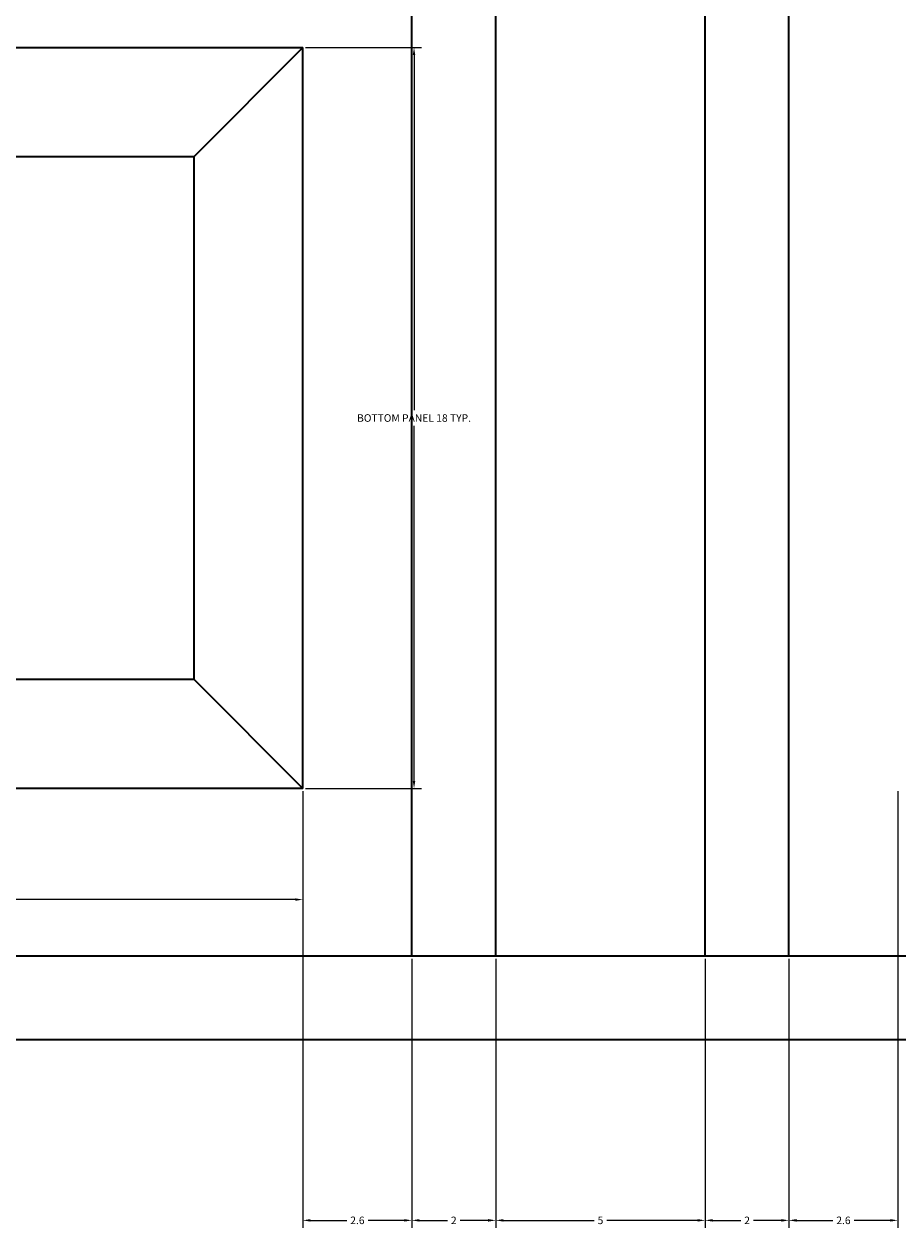
# Model space of a CAD drawing. Units: inches. Extents: x 3137 to 3299, y 1994 to 2089.
# Tile 9 of 14: x 3251 to 3272, y 1996 to 2024. Entities that reach past the tile are written whole.
import ezdxf

# ---------------------------------------------------------------- set-up
doc = ezdxf.new("R2010")
doc.units = ezdxf.units.IN
doc.header["$MEASUREMENT"] = 0
doc.layers.add('A-ANNO-DIMS', color=2, linetype='Continuous', lineweight=18)
doc.layers.add('A-DOOR', color=4, linetype='Continuous', lineweight=35)
doc.styles.get("Standard").update_dxf_attribs({"font": 'arial.ttf'})
doc.dimstyles.get("Standard").update_dxf_attribs({"dimtxt": 0.18, "dimasz": 0.18, "dimexe": 0.18, "dimexo": 0.0625, "dimgap": 0.09, "dimtad": 0, "dimtih": 1, "dimtoh": 1, "dimdec": 4, "dimzin": 0, "dimdsep": 46, "dimtxsty": 'Standard', "dimcen": 0.09, "dimadec": 0, "dimazin": 0, "dimtfac": 1, "dimtdec": 4, "dimtofl": 0, "dimtmove": 0, "dimatfit": 3, "dimfxl": 1, "dimtolj": 1, "dimtzin": 0, "dimarcsym": 0})

# ---------------------------------------------------------------- blocks, each defined once
blk = doc.blocks.new('DOOR-PANEL-RAISED-BOT')
for p, q in [((0, 17.675), (16.9, 17.675)), ((2.6, 15.075), (0, 17.675)), ((14.3, 15.075), (16.9, 17.675)), ((16.9, 0), (16.9, 17.675)), ((2.6, 15.075), (14.3, 15.075)), ((14.3, 2.6), (14.3, 15.075)), ((2.6, 2.6), (0, 0)), ((14.3, 2.6), (16.9, 0))]:
    blk.add_line(p, q)
for points in [[(16.9, 0), (0, 0), (0, 17.675)], [(14.3, 2.6), (2.6, 2.6), (2.6, 15.075)]]:
    blk.add_lwpolyline(points)
blk = doc.blocks.new('*D9')
at = {"layer": 'A-ANNO-DIMS', "color": 0, "lineweight": -2, "transparency": 16777216}
for p, q in [((3257.466, 2023.851), (3260.235, 2023.851)), ((3260.055, 2023.671), (3260.055, 2015.197)), ((3260.055, 2006.356), (3260.055, 2014.83)), ((3257.466, 2006.176), (3260.235, 2006.176))]:
    blk.add_line(p, q, dxfattribs=at)
at = {"layer": 'A-ANNO-DIMS', "color": 0, "transparency": 16777216}
for points in [[(3260.025, 2023.671), (3260.085, 2023.671), (3260.055, 2023.851)], [(3260.025, 2006.356), (3260.085, 2006.356), (3260.055, 2006.176)]]:
    blk.add_solid(points, dxfattribs=at)
at = {"layer": 'Defpoints', "color": 0, "transparency": 16777216}
for p in [(3257.404, 2023.851), (3260.055, 2023.851), (3257.404, 2006.176)]:
    blk.add_point(p, dxfattribs=at)
at = {"layer": 'A-ANNO-DIMS', "color": 0, "transparency": 16777216, "insert": (3260.055, 2015.013), "char_height": 0.18, "attachment_point": 5}
blk.add_mtext('\\A1;BOTTOM PANEL 18 TYP.', dxfattribs=at)
blk = doc.blocks.new('*D10')
at = {"layer": 'A-ANNO-DIMS', "color": 0, "lineweight": -2, "transparency": 16777216}
for p, q in [((3240.504, 2006.113), (3240.504, 2003.344)), ((3257.404, 2006.113), (3257.404, 2003.344)), ((3240.684, 2003.524), (3248.434, 2003.524)), ((3257.224, 2003.524), (3249.474, 2003.524))]:
    blk.add_line(p, q, dxfattribs=at)
at = {"layer": 'A-ANNO-DIMS', "color": 0, "transparency": 16777216}
for points in [[(3240.684, 2003.554), (3240.684, 2003.494), (3240.504, 2003.524)], [(3257.224, 2003.554), (3257.224, 2003.494), (3257.404, 2003.524)]]:
    blk.add_solid(points, dxfattribs=at)
at = {"layer": 'Defpoints', "color": 0, "transparency": 16777216}
for p in [(3240.504, 2006.176), (3257.404, 2006.176), (3257.404, 2003.524)]:
    blk.add_point(p, dxfattribs=at)
at = {"layer": 'A-ANNO-DIMS', "color": 0, "transparency": 16777216, "insert": (3248.954, 2003.524), "char_height": 0.18, "attachment_point": 5}
blk.add_mtext('\\A1;17 TYP.', dxfattribs=at)
blk = doc.blocks.new('*D59')
at = {"layer": 'A-ANNO-DIMS', "color": 0, "lineweight": -2, "transparency": 16777216}
for p, q in [((3257.404, 2006.113), (3257.404, 1995.691)), ((3260.004, 2002.113), (3260.004, 1995.691)), ((3257.584, 1995.871), (3258.449, 1995.871)), ((3259.824, 1995.871), (3258.959, 1995.871))]:
    blk.add_line(p, q, dxfattribs=at)
at = {"layer": 'A-ANNO-DIMS', "color": 0, "transparency": 16777216}
for points in [[(3257.584, 1995.901), (3257.584, 1995.841), (3257.404, 1995.871)], [(3259.824, 1995.901), (3259.824, 1995.841), (3260.004, 1995.871)]]:
    blk.add_solid(points, dxfattribs=at)
at = {"layer": 'Defpoints', "color": 0, "transparency": 16777216}
for p in [(3257.404, 2006.176), (3260.004, 2002.176), (3260.004, 1995.871)]:
    blk.add_point(p, dxfattribs=at)
at = {"layer": 'A-ANNO-DIMS', "color": 0, "transparency": 16777216, "insert": (3258.704, 1995.871), "char_height": 0.18, "attachment_point": 5}
blk.add_mtext('\\A1;2.6', dxfattribs=at)
blk = doc.blocks.new('*D60')
at = {"layer": 'A-ANNO-DIMS', "color": 0, "lineweight": -2, "transparency": 16777216}
for p, q in [((3260.004, 2002.113), (3260.004, 1995.691)), ((3262.004, 2002.113), (3262.004, 1995.691)), ((3260.184, 1995.871), (3260.854, 1995.871)), ((3261.824, 1995.871), (3261.154, 1995.871))]:
    blk.add_line(p, q, dxfattribs=at)
at = {"layer": 'A-ANNO-DIMS', "color": 0, "transparency": 16777216}
for points in [[(3260.184, 1995.901), (3260.184, 1995.841), (3260.004, 1995.871)], [(3261.824, 1995.901), (3261.824, 1995.841), (3262.004, 1995.871)]]:
    blk.add_solid(points, dxfattribs=at)
at = {"layer": 'Defpoints', "color": 0, "transparency": 16777216}
for p in [(3260.004, 2002.176), (3262.004, 2002.176), (3262.004, 1995.871)]:
    blk.add_point(p, dxfattribs=at)
at = {"layer": 'A-ANNO-DIMS', "color": 0, "transparency": 16777216, "insert": (3261.004, 1995.871), "char_height": 0.18, "attachment_point": 5}
blk.add_mtext('\\A1;2', dxfattribs=at)
blk = doc.blocks.new('*D61')
at = {"layer": 'A-ANNO-DIMS', "color": 0, "lineweight": -2, "transparency": 16777216}
for p, q in [((3262.004, 2002.113), (3262.004, 1995.691)), ((3267.004, 2002.113), (3267.004, 1995.691)), ((3262.184, 1995.871), (3264.354, 1995.871)), ((3266.824, 1995.871), (3264.654, 1995.871))]:
    blk.add_line(p, q, dxfattribs=at)
at = {"layer": 'A-ANNO-DIMS', "color": 0, "transparency": 16777216}
for points in [[(3262.184, 1995.901), (3262.184, 1995.841), (3262.004, 1995.871)], [(3266.824, 1995.901), (3266.824, 1995.841), (3267.004, 1995.871)]]:
    blk.add_solid(points, dxfattribs=at)
at = {"layer": 'Defpoints', "color": 0, "transparency": 16777216}
for p in [(3262.004, 2002.176), (3267.004, 2002.176), (3267.004, 1995.871)]:
    blk.add_point(p, dxfattribs=at)
at = {"layer": 'A-ANNO-DIMS', "color": 0, "transparency": 16777216, "insert": (3264.504, 1995.871), "char_height": 0.18, "attachment_point": 5}
blk.add_mtext('\\A1;5', dxfattribs=at)
blk = doc.blocks.new('*D62')
at = {"layer": 'A-ANNO-DIMS', "color": 0, "lineweight": -2, "transparency": 16777216}
for p, q in [((3267.004, 2002.113), (3267.004, 1995.691)), ((3269.004, 2002.113), (3269.004, 1995.691)), ((3267.184, 1995.871), (3267.854, 1995.871)), ((3268.824, 1995.871), (3268.154, 1995.871))]:
    blk.add_line(p, q, dxfattribs=at)
at = {"layer": 'A-ANNO-DIMS', "color": 0, "transparency": 16777216}
for points in [[(3267.184, 1995.901), (3267.184, 1995.841), (3267.004, 1995.871)], [(3268.824, 1995.901), (3268.824, 1995.841), (3269.004, 1995.871)]]:
    blk.add_solid(points, dxfattribs=at)
at = {"layer": 'Defpoints', "color": 0, "transparency": 16777216}
for p in [(3267.004, 2002.176), (3269.004, 2002.176), (3269.004, 1995.871)]:
    blk.add_point(p, dxfattribs=at)
at = {"layer": 'A-ANNO-DIMS', "color": 0, "transparency": 16777216, "insert": (3268.004, 1995.871), "char_height": 0.18, "attachment_point": 5}
blk.add_mtext('\\A1;2', dxfattribs=at)
blk = doc.blocks.new('*D63')
at = {"layer": 'A-ANNO-DIMS', "color": 0, "lineweight": -2, "transparency": 16777216}
for p, q in [((3271.604, 2006.113), (3271.604, 1995.691)), ((3269.004, 2002.113), (3269.004, 1995.691)), ((3269.184, 1995.871), (3270.049, 1995.871)), ((3271.424, 1995.871), (3270.559, 1995.871))]:
    blk.add_line(p, q, dxfattribs=at)
at = {"layer": 'A-ANNO-DIMS', "color": 0, "transparency": 16777216}
for points in [[(3269.184, 1995.901), (3269.184, 1995.841), (3269.004, 1995.871)], [(3271.424, 1995.901), (3271.424, 1995.841), (3271.604, 1995.871)]]:
    blk.add_solid(points, dxfattribs=at)
at = {"layer": 'Defpoints', "color": 0, "transparency": 16777216}
for p in [(3271.604, 2006.176), (3269.004, 2002.176), (3271.604, 1995.871)]:
    blk.add_point(p, dxfattribs=at)
at = {"layer": 'A-ANNO-DIMS', "color": 0, "transparency": 16777216, "insert": (3270.304, 1995.871), "char_height": 0.18, "attachment_point": 5}
blk.add_mtext('\\A1;2.6', dxfattribs=at)

msp = doc.modelspace()

# ---------------------------------------------------------------- linework, layer by layer
at = {"layer": 'A-DOOR'}
for p, q in [((3260.0039, 2002.1756), (3260.0039, 2028.6759)), ((3262.0039, 2002.1756), (3262.0039, 2028.6759)), ((3267.0039, 2002.1756), (3267.0039, 2028.6759)), ((3269.0039, 2002.1756), (3269.0039, 2028.6759))]:
    msp.add_line(p, q, dxfattribs=at)
for points in [[(3234.5039, 2084.1756), (3294.5039, 2084.1756), (3294.5039, 2000.1756), (3234.5039, 2000.1756)], [(3236.5039, 2082.1756), (3292.5039, 2082.1756), (3292.5039, 2002.1756), (3236.5039, 2002.1756)]]:
    msp.add_lwpolyline(points, close=True, dxfattribs=at)

# ---------------------------------------------------------------- block references
msp.add_blockref('DOOR-PANEL-RAISED-BOT', (3240.504, 2006.176), dxfattribs=at)

# ---------------------------------------------------------------- dimensions: what is measured, and where the dimension line sits
at = {"layer": 'A-ANNO-DIMS'}
dim = msp.add_linear_dim(base=(3260.0553, 2023.8512), p1=(3257.4039, 2006.1756), p2=(3257.4039, 2023.8512), angle=90, text='BOTTOM PANEL <> TYP.', dimstyle='Standard', override={"dimdec": 0, "dimrnd": 0, "dimzin": 0, "dimlunit": 2}, dxfattribs=at)
dim.commit()
dim.dimension.update_dxf_attribs({"geometry": '*D9', "text_midpoint": (3260.0553, 2015.0134)})
dim = msp.add_linear_dim(base=(3257.4039, 2003.5243), p1=(3240.5039, 2006.1756), p2=(3257.4039, 2006.1756), text='<> TYP.', dimstyle='Standard', override={"dimdec": 0, "dimrnd": 0, "dimzin": 0, "dimlunit": 2}, dxfattribs=at)
dim.commit()
dim.dimension.update_dxf_attribs({"geometry": '*D10', "text_midpoint": (3248.9539, 2003.5243)})
for base, p1, p2, override, picture, middle in [((3260.0039, 1995.8706), (3257.4039, 2006.1756), (3260.0039, 2002.1756), {"dimdec": 1, "dimlfac": 1, "dimrnd": 0, "dimzin": 0, "dimdsep": 46, "dimlunit": 2}, '*D59', (3258.7039, 1995.8706)), ((3271.6039, 1995.8706), (3269.0039, 2002.1756), (3271.6039, 2006.1756), {"dimdec": 1, "dimlfac": 1, "dimrnd": 0, "dimzin": 0, "dimdsep": 46, "dimlunit": 2}, '*D63', (3270.3039, 1995.8706)), ((3262.0039, 1995.8706), (3260.0039, 2002.1756), (3262.0039, 2002.1756), {"dimdec": 0, "dimlfac": 1, "dimrnd": 0, "dimzin": 0, "dimdsep": 46, "dimlunit": 2}, '*D60', (3261.0039, 1995.8706)), ((3267.0039, 1995.8706), (3262.0039, 2002.1756), (3267.0039, 2002.1756), {"dimdec": 0, "dimlfac": 1, "dimrnd": 0, "dimzin": 0, "dimdsep": 46, "dimlunit": 2}, '*D61', (3264.5039, 1995.8706)), ((3269.0039, 1995.8706), (3267.0039, 2002.1756), (3269.0039, 2002.1756), {"dimdec": 0, "dimlfac": 1, "dimrnd": 0, "dimzin": 0, "dimdsep": 46, "dimlunit": 2}, '*D62', (3268.0039, 1995.8706))]:
    dim = msp.add_linear_dim(base=base, p1=p1, p2=p2, dimstyle='Standard', override=override, dxfattribs=at)
    dim.commit()
    dim.dimension.update_dxf_attribs({"geometry": picture, "text_midpoint": middle})

doc.saveas('drawing.dxf')
